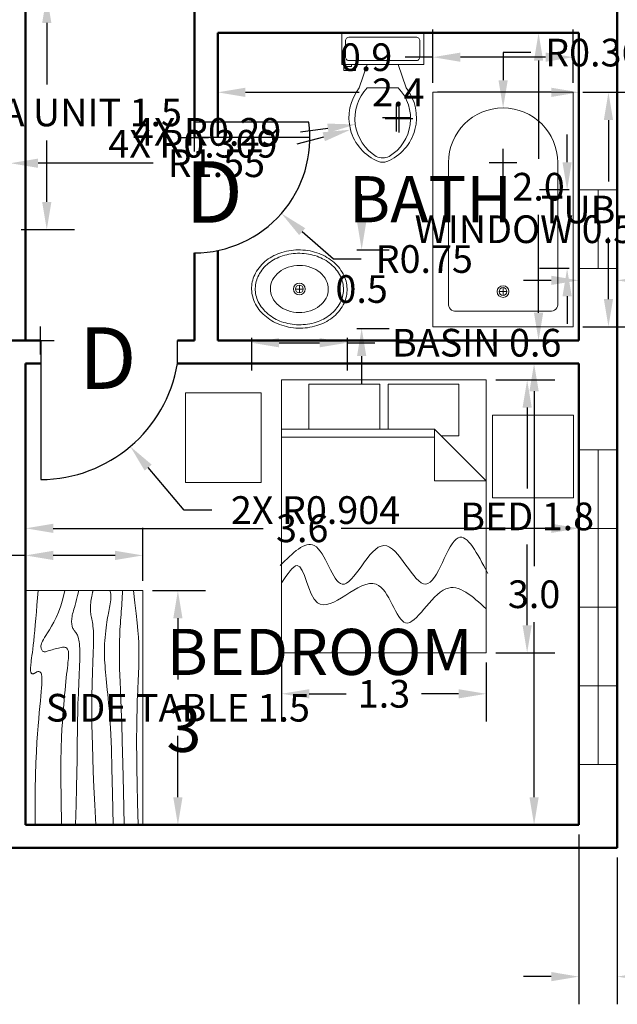
# Model space of a CAD drawing. Units: metres. Extents: x 3.9 to 21.3, y 24.8 to 56.5.
# Tile 2 of 6: x 11.9 to 15.8, y 24.8 to 31.2. Entities that reach past the tile are written whole.
import ezdxf

# ---------------------------------------------------------------- set-up
doc = ezdxf.new("R2010")
doc.units = ezdxf.units.M
doc.header["$MEASUREMENT"] = 0
for name, color, linetype, lineweight in [('A-AREA-IDEN', 3, 'Continuous', 25), ('A-FLOR-FIXT', 9, 'Continuous', 18), ('DIMENSIONS', 2, 'Continuous', 18), ('DOOR', 5, 'Continuous', 25), ('FURNITURE', 6, 'Continuous', 18), ('TEXT', 3, 'Continuous', 18), ('WALL', 1, 'Continuous', 50), ('WINDOW', 4, 'Continuous', 18)]:
    doc.layers.add(name, color=color, linetype=linetype, lineweight=lineweight)
doc.styles.get("Standard").update_dxf_attribs({"font": 'arial.ttf'})
doc.dimstyles.get("Standard").update_dxf_attribs({"dimtxt": 0.18, "dimasz": 0.18, "dimexe": 0.18, "dimexo": 0.0625, "dimgap": 0.09, "dimtad": 0, "dimtih": 1, "dimtoh": 1, "dimdec": 1, "dimzin": 0, "dimdsep": 46, "dimtxsty": 'Standard', "dimcen": 0.09, "dimadec": 0, "dimazin": 0, "dimtfac": 1, "dimtdec": 1, "dimtofl": 0, "dimtmove": 0, "dimatfit": 3, "dimfxl": 1, "dimtolj": 1, "dimtzin": 0, "dimarcsym": 0})

# ---------------------------------------------------------------- blocks, each defined once
blk = doc.blocks.new('Toilet - top')
for p, q in [((9.5, -6), (9.5, -2)), ((-10, -8.5), (-8, -8.5)), ((-10, -9.5), (-10, -8.5)), ((-7, -9.5), (-10, -9.5)), ((-8, -8.5), (-8, -8)), ((-7, -8), (-7, -9.5)), ((-4, -8), (-6, -14)), ((4, -8), (6, -14)), ((4, -14), (-4, -14))]:
    blk.add_line(p, q)
blk.add_lwpolyline([(10.5, -8), (10.5, 0), (-10.5, 0), (-10.5, -8)], close=True)
for points in [[(-9.5, -2), (-9.5, -6)], [(8.5, -1), (-8.5, -1)], [(-8.5, -7), (8.5, -7)]]:
    blk.add_lwpolyline(points)
for centre, radius, start, end in [((-8.62, -1.88), 0.884, 81.8699, 188.1301), ((8.62, -1.88), 0.884, 351.8699, 98.1301), ((-8.62, -6.12), 0.884, 171.8699, 278.1301), ((8.62, -6.12), 0.884, 261.8699, 8.1301), ((3.52, -21.58), 12.17, 141.4691, 247.9714), ((4.2, -21.82), 11.33, 136.3677, 238.9468), ((-3.52, -21.58), 12.17, 292.0284, 38.5307), ((-4.2, -21.82), 11.33, 301.053, 43.6321), ((0, -27.88), 4, 245.7318, 294.2682), ((0, -29), 4, 254.8605, 285.1395)]:
    blk.add_arc(centre, radius, start, end)
blk = doc.blocks.new('Bath Tub - 26 x 60 in.')
for p, q in [((9, -17), (9, -19)), ((8, -18), (10, -18))]:
    blk.add_line(p, q)
blk.add_lwpolyline([(0, -36), (0, 0), (60, 0), (60, -36)], close=True)
for points in [[(6, -4), (42, -4)], [(4, -30), (4, -6)], [(42, -32), (6, -32)]]:
    blk.add_lwpolyline(points)
for radius in [1.5, 1]:
    blk.add_circle((9, -18), radius)
for centre, radius, start, end in [((5.75, -5.75), 1.77, 81.8699, 188.1301), ((42, -18), 14, 270, 90), ((5.75, -30.25), 1.77, 171.8699, 278.1301)]:
    blk.add_arc(centre, radius, start, end)
blk = doc.blocks.new('Sink - Oval top')
for p, q in [((-1, 0), (1, 0)), ((0, 1), (0, -1))]:
    blk.add_line(p, q)
for points in [[(-12.23, 0.39, 0.117634), (-11.46, -3.36, 0.104469), (-8.88, -6.8, 0.090016), (-5.08, -9.07, 0.08192), (-0.32, -10.02, 0.08192), (4.49, -9.38, 0.090016), (8.42, -7.36, 0.104469), (11.22, -4.09, 0.117634), (12.23, -0.39, 0.117634), (11.46, 3.36, 0.104469), (8.88, 6.8, 0.090016), (5.08, 9.07, 0.08192), (0.32, 10.02, 0.08192), (-4.49, 9.38, 0.090016), (-8.42, 7.36, 0.104469), (-11.22, 4.09, 0.117634)], [(-11.29, 0.16, 0.118622), (-10.52, -3.25, 0.104678), (-8.07, -6.36, 0.089562), (-4.54, -8.37, 0.081185), (-0.13, -9.15, 0.081185), (4.3, -8.49, 0.089562), (7.89, -6.58, 0.104678), (10.42, -3.55, 0.118622), (11.29, -0.16, 0.118622), (10.52, 3.25, 0.104678), (8.07, 6.36, 0.089562), (4.54, 8.37, 0.081185), (0.13, 9.15, 0.081185), (-4.3, 8.49, 0.089562), (-7.89, 6.58, 0.104678), (-10.42, 3.55, 0.118622)], [(-7.42, 0.08, 0.118283), (-6.91, -2.17, 0.104607), (-5.29, -4.21, 0.089718), (-2.97, -5.53, 0.081436), (-0.07, -6.04, 0.081436), (2.84, -5.59, 0.089718), (5.2, -4.33, 0.104607), (6.86, -2.32, 0.118283), (7.42, -0.08, 0.118283), (6.91, 2.17, 0.104607), (5.29, 4.21, 0.089718), (2.97, 5.53, 0.081436), (0.07, 6.04, 0.081436), (-2.84, 5.59, 0.089718), (-5.2, 4.33, 0.104607), (-6.86, 2.32, 0.118283)]]:
    blk.add_lwpolyline(points, format="xyb", close=True)
for radius in [1.5, 1]:
    blk.add_circle((0, 0), radius)
blk = doc.blocks.new('Bed - Queen')
for p, q in [((0, -80.00003), (0, 0)), ((0, 0), (59.99999, 0)), ((59.99999, 0), (59.99999, -80.00003)), ((7.99999, -1.2), (28.79998, -1.2)), ((7.99999, -14.4), (7.99999, -1.2)), ((28.79998, -1.2), (28.79998, -14.4)), ((31.19999, -1.2), (51.99999, -1.2)), ((31.19999, -14.4), (31.19999, -1.2)), ((51.99999, -1.2), (51.99999, -16.4)), ((0, -14.4), (44.8, -14.4)), ((59.99999, -29.6), (44.8, -14.4)), ((44.8, -14.4), (44.8, -29.6)), ((44.8, -16.8), (0, -16.8)), ((51.99999, -16.4), (46.79936, -16.4)), ((44.8, -29.6), (59.99999, -29.6)), ((59.99999, -80.00003), (0, -80.00003))]:
    blk.add_line(p, q)
blk = doc.blocks.new('Table - Rectangular Woodgrain 60 x 30 in.')
for p, q in [((0, 0), (0, -30)), ((60, 0), (0, 0)), ((60, -30), (60, 0)), ((0, -30), (60, -30))]:
    blk.add_line(p, q)
for points in [[(0, -2.4), (4.8155, -2.418), (9.0302, -2.4688), (12.709, -2.5477), (15.9167, -2.65), (18.7181, -2.7711), (21.1781, -2.9063), (23.3616, -3.0508), (25.3333, -3.2), (27.1477, -3.3495), (28.8172, -3.4958), (30.3437, -3.636), (31.7291, -3.7667), (32.9756, -3.8849), (34.0849, -3.9875), (35.059, -4.0714), (35.9, -4.1334), (36.6114, -4.1711), (37.2041, -4.1854), (37.6906, -4.1779), (38.0833, -4.15), (38.3948, -4.1034), (38.6375, -4.0396), (38.8239, -3.9602), (38.9666, -3.8667), (39.0764, -3.7608), (39.1573, -3.6448), (39.2116, -3.521), (39.2416, -3.3917), (39.2498, -3.2593), (39.2385, -3.1261), (39.21, -2.9944), (39.1666, -2.8667), (39.111, -2.7447), (39.0468, -2.6281), (38.978, -2.5163), (38.9083, -2.4083), (38.8418, -2.3035), (38.7823, -2.201), (38.7337, -2.1001), (38.7, -2), (38.6844, -1.9003), (38.6875, -1.8021), (38.7094, -1.707), (38.75, -1.6167), (38.8094, -1.5326), (38.8875, -1.4563), (38.9844, -1.3893), (39.1, -1.3333), (39.2351, -1.2896), (39.3937, -1.2583), (39.5804, -1.2396), (39.8, -1.2333), (40.057, -1.2396), (40.3562, -1.2583), (40.7023, -1.2896), (41.1, -1.3333), (41.5547, -1.3895), (42.0755, -1.4573), (42.6721, -1.5361), (43.3542, -1.625), (44.1316, -1.7233), (45.014, -1.8302), (46.0114, -1.9449), (47.1333, -2.0667), (48.3862, -2.1947), (49.7625, -2.3281), (51.2513, -2.4663), (52.8416, -2.6083), (54.5226, -2.7535), (56.2833, -2.9011), (58.1127, -3.0501), (60, -3.2)], [(0, -9.2), (6.5759, -9.0858), (11.9385, -9.0365), (16.2527, -9.0418), (19.6833, -9.0917), (22.3952, -9.1759), (24.5531, -9.2844), (26.322, -9.4069), (27.8666, -9.5333), (29.3241, -9.6553), (30.7203, -9.7719), (32.0532, -9.8837), (33.3208, -9.9917), (34.5213, -10.0965), (35.6526, -10.199), (36.7128, -10.2999), (37.7, -10.4), (38.6129, -10.4996), (39.4531, -10.5969), (40.223, -10.6895), (40.925, -10.775), (41.5613, -10.8512), (42.1344, -10.9156), (42.6465, -10.966), (43.1, -11), (43.4976, -11.0158), (43.8437, -11.0136), (44.143, -10.9942), (44.4, -10.9583), (44.6195, -10.9069), (44.8062, -10.8406), (44.9648, -10.7603), (45.1, -10.6667), (45.2155, -10.5598), (45.3114, -10.4365), (45.3871, -10.2929), (45.4416, -10.125), (45.4743, -9.929), (45.4844, -9.7011), (45.4709, -9.4371), (45.4333, -9.1333), (45.3716, -8.7883), (45.2896, -8.4104), (45.1919, -8.0107), (45.0833, -7.6), (44.9685, -7.1893), (44.8521, -6.7896), (44.7388, -6.4117), (44.6333, -6.0667), (44.54, -5.7628), (44.4614, -5.4979), (44.4001, -5.2675), (44.3583, -5.0667), (44.3384, -4.8909), (44.3427, -4.7354), (44.3736, -4.5956), (44.4333, -4.4667), (44.5236, -4.3453), (44.6427, -4.2333), (44.7884, -4.1339), (44.9583, -4.05), (45.1501, -3.9849), (45.3614, -3.9417), (45.59, -3.9234), (45.8333, -3.9333), (46.0915, -3.9749), (46.3734, -4.0531), (46.6906, -4.1736), (47.0542, -4.3417), (47.4756, -4.5629), (47.9661, -4.8427), (48.5372, -5.1866), (49.2, -5.6), (49.9676, -6.0844), (50.8594, -6.625), (51.8965, -7.2031), (53.1, -7.8), (54.491, -8.3969), (56.0906, -8.975), (57.9199, -9.5156), (60, -10)], [(0, -12.8), (5.1847, -12.9322), (9.6213, -13.0323), (13.3963, -13.1059), (16.5958, -13.1583), (19.3063, -13.1952), (21.614, -13.2219), (23.6054, -13.2439), (25.3666, -13.2667), (26.9728, -13.2947), (28.4531, -13.3281), (29.8256, -13.3663), (31.1083, -13.4083), (32.3191, -13.4535), (33.476, -13.501), (34.597, -13.5501), (35.7, -13.6), (36.7984, -13.6497), (37.8875, -13.6979), (38.9578, -13.743), (40, -13.7833), (41.0047, -13.8174), (41.9625, -13.8438), (42.864, -13.8607), (43.7, -13.8667), (44.4631, -13.8604), (45.1552, -13.8417), (45.7801, -13.8104), (46.3416, -13.7667), (46.8439, -13.7104), (47.2906, -13.6417), (47.6858, -13.5604), (48.0333, -13.4667), (48.3375, -13.3608), (48.6042, -13.2448), (48.8396, -13.121), (49.05, -12.9917), (49.2417, -12.8593), (49.4208, -12.7261), (49.5937, -12.5944), (49.7667, -12.4667), (49.9452, -12.3451), (50.1323, -12.2313), (50.3303, -12.1268), (50.5416, -12.0333), (50.7686, -11.9524), (51.0135, -11.8854), (51.2788, -11.8341), (51.5666, -11.8), (51.8785, -11.7843), (52.2116, -11.7865), (52.562, -11.8059), (52.926, -11.8417), (53.2998, -11.8931), (53.6795, -11.9594), (54.0614, -12.0397), (54.4416, -12.1333), (54.8223, -12.2401), (55.2293, -12.3625), (55.6942, -12.5037), (56.2489, -12.6667), (56.9251, -12.8547), (57.7545, -13.0708), (58.7689, -13.3182), (60, -13.6)], [(0, -18), (5.124, -17.7273), (9.6609, -17.5057), (13.6705, -17.3303), (17.2125, -17.1958), (20.3467, -17.0973), (23.1328, -17.0297), (25.6307, -16.9878), (27.9, -16.9667), (29.9928, -16.9617), (31.9302, -16.9703), (33.7254, -16.9907), (35.3917, -17.0208), (36.9423, -17.0588), (38.3906, -17.1026), (39.7499, -17.1503), (41.0333, -17.2), (42.2519, -17.2496), (43.4073, -17.2969), (44.4986, -17.3395), (45.525, -17.375), (46.4858, -17.4012), (47.3802, -17.4156), (48.2074, -17.416), (48.9667, -17.4), (49.6583, -17.3662), (50.2872, -17.3167), (50.8595, -17.2547), (51.3812, -17.1833), (51.8584, -17.1057), (52.2971, -17.025), (52.7034, -16.9443), (53.0833, -16.8667), (53.443, -16.7951), (53.789, -16.7313), (54.128, -16.6768), (54.4666, -16.6334), (54.8115, -16.6024), (55.1693, -16.5854), (55.5465, -16.5841), (55.95, -16.6), (56.3828, -16.6337), (56.8346, -16.6823), (57.2915, -16.7418), (57.7396, -16.8084), (58.165, -16.878), (58.5539, -16.9469), (58.8924, -17.0111), (59.1666, -17.0667), (59.3679, -17.1107), (59.5078, -17.1438), (59.6032, -17.1675), (59.6708, -17.1833), (59.7275, -17.193), (59.7901, -17.1979), (59.8753, -17.1998), (60, -17.2)], [(0, -22.4), (8.0098, -22.2501), (14.4094, -22.1011), (19.4168, -21.9535), (23.25, -21.8083), (26.1269, -21.6663), (28.2656, -21.5281), (29.884, -21.3947), (31.2, -21.2667), (32.3967, -21.1448), (33.5172, -21.0292), (34.5697, -20.9198), (35.5625, -20.8167), (36.5037, -20.7198), (37.4015, -20.6292), (38.2642, -20.5448), (39.1, -20.4667), (39.9164, -20.3951), (40.7187, -20.3313), (41.5117, -20.2768), (42.3, -20.2333), (43.0883, -20.2024), (43.8812, -20.1854), (44.6836, -20.1841), (45.5, -20.2), (46.3328, -20.234), (47.1747, -20.2844), (48.0163, -20.3488), (48.8479, -20.425), (49.66, -20.5106), (50.4429, -20.6031), (51.1872, -20.7004), (51.8833, -20.8), (52.5246, -20.8999), (53.1166, -20.9995), (53.6681, -21.0983), (54.1875, -21.1958), (54.6834, -21.2919), (55.1646, -21.3859), (55.6394, -21.4777), (56.1167, -21.5667), (56.6028, -21.6515), (57.0961, -21.7266), (57.5929, -21.7852), (58.0896, -21.8208), (58.5823, -21.8268), (59.0674, -21.7964), (59.5412, -21.723), (60, -21.6)], [(0, -25.2), (8.6355, -25.0504), (15.7026, -24.9031), (21.4049, -24.7606), (25.9458, -24.625), (29.529, -24.4988), (32.3578, -24.3844), (34.6359, -24.284), (36.5667, -24.2), (38.3213, -24.1341), (39.9417, -24.0854), (41.437, -24.0523), (42.8167, -24.0333), (44.0901, -24.0268), (45.2667, -24.0313), (46.3557, -24.0451), (47.3667, -24.0667), (48.309, -24.0947), (49.1928, -24.1287), (50.0284, -24.168), (50.826, -24.2125), (51.5959, -24.2617), (52.3483, -24.3151), (53.0935, -24.3725), (53.8417, -24.4334), (54.6009, -24.497), (55.3699, -24.561), (56.1454, -24.6226), (56.9239, -24.6792), (57.7021, -24.7279), (58.4764, -24.7662), (59.2435, -24.7911), (60, -24.8)], [(0, -28.8), (5.6867, -28.6681), (10.45, -28.5698), (14.407, -28.5012), (17.675, -28.4584), (20.3711, -28.4374), (22.6125, -28.4344), (24.5164, -28.4455), (26.2, -28.4667), (27.762, -28.4947), (29.2276, -28.5281), (30.6033, -28.5663), (31.8958, -28.6084), (33.1118, -28.6535), (34.2578, -28.7011), (35.3405, -28.7501), (36.3666, -28.8), (37.3443, -28.8497), (38.288, -28.8974), (39.2137, -28.9412), (40.1375, -28.9792), (41.0753, -29.0093), (42.0432, -29.0297), (43.0572, -29.0384), (44.1333, -29.0333), (45.2936, -29.0114), (46.5843, -28.9641), (48.0579, -28.8816), (49.7666, -28.7542), (51.7629, -28.5721), (54.0989, -28.3255), (56.8272, -28.0048), (60, -27.6)]]:
    blk.add_lwpolyline(points)
blk = doc.blocks.new('*D21')
at = {"layer": 'Defpoints', "color": 0, "transparency": 16777216}
for p in [(15.7571, 38.8951), (15.7571, 25.8451), (17.2883, 25.8451)]:
    blk.add_point(p, dxfattribs=at)
at = {"layer": 'DIMENSIONS', "color": 0, "lineweight": -2, "transparency": 16777216}
for p, q in [((15.8196, 38.8951), (17.4683, 38.8951)), ((17.2883, 38.7151), (17.2883, 32.8688)), ((17.2883, 26.0251), (17.2883, 31.8713)), ((15.8196, 25.8451), (17.4683, 25.8451))]:
    blk.add_line(p, q, dxfattribs=at)
at = {"layer": 'DIMENSIONS', "color": 0, "transparency": 16777216}
for points in [[(17.2583, 38.7151), (17.3183, 38.7151), (17.2883, 38.8951)], [(17.2583, 26.0251), (17.3183, 26.0251), (17.2883, 25.8451)]]:
    blk.add_solid(points, dxfattribs=at)
at = {"layer": 'DIMENSIONS', "color": 0, "transparency": 16777216, "insert": (17.2883, 32.3701), "char_height": 0.18, "attachment_point": 5}
blk.add_mtext('\\A1;{\\H4.44444x;13.1}', dxfattribs=at)
blk = doc.blocks.new('*D30')
at = {"layer": 'Defpoints', "color": 0, "transparency": 16777216}
for p in [(13.8962, 31.1451), (13.9549, 29.1451), (15.2447, 29.1451)]:
    blk.add_point(p, dxfattribs=at)
at = {"layer": 'DIMENSIONS', "color": 0, "lineweight": -2, "transparency": 16777216}
for p, q in [((13.9587, 31.1451), (15.4247, 31.1451)), ((15.2447, 30.9651), (15.2447, 30.327)), ((15.2447, 29.3251), (15.2447, 29.9632)), ((14.0174, 29.1451), (15.4247, 29.1451))]:
    blk.add_line(p, q, dxfattribs=at)
at = {"layer": 'DIMENSIONS', "color": 0, "transparency": 16777216}
for points in [[(15.2147, 30.9651), (15.2747, 30.9651), (15.2447, 31.1451)], [(15.2147, 29.3251), (15.2747, 29.3251), (15.2447, 29.1451)]]:
    blk.add_solid(points, dxfattribs=at)
at = {"layer": 'DIMENSIONS', "color": 0, "transparency": 16777216, "insert": (15.2447, 30.1451), "char_height": 0.18, "attachment_point": 5}
blk.add_mtext('\\A1;2.0', dxfattribs=at)
blk = doc.blocks.new('*D31')
at = {"layer": 'Defpoints', "color": 0, "transparency": 16777216}
for p in [(13.1571, 31.1451), (15.5071, 31.1451), (15.5071, 30.7589)]:
    blk.add_point(p, dxfattribs=at)
at = {"layer": 'DIMENSIONS', "color": 0, "lineweight": -2, "transparency": 16777216}
for p, q in [((13.1571, 31.0826), (13.1571, 30.5789)), ((15.5071, 31.0826), (15.5071, 30.5789)), ((13.3371, 30.7589), (14.0771, 30.7589)), ((15.3271, 30.7589), (14.5871, 30.7589))]:
    blk.add_line(p, q, dxfattribs=at)
at = {"layer": 'DIMENSIONS', "color": 0, "transparency": 16777216}
for points in [[(13.3371, 30.7889), (13.3371, 30.7289), (13.1571, 30.7589)], [(15.3271, 30.7889), (15.3271, 30.7289), (15.5071, 30.7589)]]:
    blk.add_solid(points, dxfattribs=at)
at = {"layer": 'DIMENSIONS', "color": 0, "transparency": 16777216, "insert": (14.3321, 30.7589), "char_height": 0.18, "attachment_point": 5}
blk.add_mtext('\\A1;2.4', dxfattribs=at)
blk = doc.blocks.new('*D32')
at = {"layer": 'Defpoints', "color": 0, "transparency": 16777216}
for p in [(15.5071, 28.9951), (15.2156, 25.9951), (15.5071, 25.9951)]:
    blk.add_point(p, dxfattribs=at)
at = {"layer": 'DIMENSIONS', "color": 0, "lineweight": -2, "transparency": 16777216}
for p, q in [((15.4446, 28.9951), (15.0356, 28.9951)), ((15.2156, 28.8151), (15.2156, 27.677)), ((15.2156, 26.1751), (15.2156, 27.3131)), ((15.4446, 25.9951), (15.0356, 25.9951))]:
    blk.add_line(p, q, dxfattribs=at)
at = {"layer": 'DIMENSIONS', "color": 0, "transparency": 16777216}
for points in [[(15.1856, 28.8151), (15.2456, 28.8151), (15.2156, 28.9951)], [(15.1856, 26.1751), (15.2456, 26.1751), (15.2156, 25.9951)]]:
    blk.add_solid(points, dxfattribs=at)
at = {"layer": 'DIMENSIONS', "color": 0, "transparency": 16777216, "insert": (15.2156, 27.4951), "char_height": 0.18, "attachment_point": 5}
blk.add_mtext('\\A1;3.0', dxfattribs=at)
blk = doc.blocks.new('*D33')
at = {"layer": 'Defpoints', "color": 0, "transparency": 16777216}
for p in [(11.9071, 27.9939), (15.5071, 27.9237), (15.5071, 27.9237)]:
    blk.add_point(p, dxfattribs=at)
at = {"layer": 'DIMENSIONS', "color": 0, "lineweight": -2, "transparency": 16777216}
for p, q in [((15.5071, 27.9862), (15.5071, 28.1037)), ((11.9071, 27.9314), (11.9071, 27.7437)), ((12.0871, 27.9237), (13.4534, 27.9237)), ((15.3271, 27.9237), (13.9609, 27.9237))]:
    blk.add_line(p, q, dxfattribs=at)
at = {"layer": 'DIMENSIONS', "color": 0, "transparency": 16777216}
for points in [[(12.0871, 27.9537), (12.0871, 27.8937), (11.9071, 27.9237)], [(15.3271, 27.9537), (15.3271, 27.8937), (15.5071, 27.9237)]]:
    blk.add_solid(points, dxfattribs=at)
at = {"layer": 'DIMENSIONS', "color": 0, "transparency": 16777216, "insert": (13.7071, 27.9237), "char_height": 0.18, "attachment_point": 5}
blk.add_mtext('\\A1;3.6', dxfattribs=at)
blk = doc.blocks.new('WIN-4-LIGHT-2046')
for p, q in [((0.5115, -0.125), (0, -0.125)), ((0.5115, -0.125), (1.0231, -0.125)), ((1.5346, -0.125), (1.0231, -0.125)), ((1.5346, -0.125), (2.0462, -0.125))]:
    blk.add_line(p, q)
for points in [[(0.5115, 0), (0, 0), (0, -0.25), (0.5115, -0.25)], [(0.5115, 0), (1.0231, 0), (1.0231, -0.25), (0.5115, -0.25)], [(1.5346, 0), (1.0231, 0), (1.0231, -0.25), (1.5346, -0.25)], [(1.5346, 0), (2.0462, 0), (2.0462, -0.25), (1.5346, -0.25)]]:
    blk.add_lwpolyline(points, close=True)
blk = doc.blocks.new('WIN-1-LIGHT-512')
blk.add_line((0, -0.125), (0.5115, -0.125))
blk.add_lwpolyline([(0, 0), (0.5115, 0), (0.5115, -0.25), (0, -0.25)], close=True)
blk = doc.blocks.new('*D43')
at = {"layer": 'Defpoints', "color": 0, "transparency": 16777216}
for p in [(14.9043, 28.8887), (15.1705, 28.8887), (14.9043, 27.1139)]:
    blk.add_point(p, dxfattribs=at)
at = {"layer": 'DIMENSIONS', "color": 0, "lineweight": -2, "transparency": 16777216}
for p, q in [((14.9668, 28.8887), (15.3505, 28.8887)), ((15.1705, 28.7087), (15.1705, 28.1832)), ((15.1705, 27.2939), (15.1705, 27.8194)), ((14.9668, 27.1139), (15.3505, 27.1139))]:
    blk.add_line(p, q, dxfattribs=at)
at = {"layer": 'DIMENSIONS', "color": 0, "transparency": 16777216}
for points in [[(15.1405, 28.7087), (15.2005, 28.7087), (15.1705, 28.8887)], [(15.1405, 27.2939), (15.2005, 27.2939), (15.1705, 27.1139)]]:
    blk.add_solid(points, dxfattribs=at)
at = {"layer": 'DIMENSIONS', "color": 0, "transparency": 16777216, "insert": (15.1705, 28.0013), "char_height": 0.18, "attachment_point": 5}
blk.add_mtext('\\A1;BED 1.8', dxfattribs=at)
blk = doc.blocks.new('*D44')
at = {"layer": 'Defpoints', "color": 0, "transparency": 16777216}
for p in [(13.5732, 27.1139), (14.9043, 27.1139), (14.9043, 26.8477)]:
    blk.add_point(p, dxfattribs=at)
at = {"layer": 'DIMENSIONS', "color": 0, "lineweight": -2, "transparency": 16777216}
for p, q in [((13.5732, 27.0514), (13.5732, 26.6677)), ((14.9043, 27.0514), (14.9043, 26.6677)), ((13.7532, 26.8477), (13.9934, 26.8477)), ((14.7243, 26.8477), (14.4841, 26.8477))]:
    blk.add_line(p, q, dxfattribs=at)
at = {"layer": 'DIMENSIONS', "color": 0, "transparency": 16777216}
for points in [[(13.7532, 26.8777), (13.7532, 26.8177), (13.5732, 26.8477)], [(14.7243, 26.8777), (14.7243, 26.8177), (14.9043, 26.8477)]]:
    blk.add_solid(points, dxfattribs=at)
at = {"layer": 'DIMENSIONS', "color": 0, "transparency": 16777216, "insert": (14.2388, 26.8477), "char_height": 0.18, "attachment_point": 5}
blk.add_mtext('\\A1;1.3', dxfattribs=at)
blk = doc.blocks.new('*D47')
at = {"layer": 'Defpoints', "color": 0, "transparency": 16777216}
for p in [(15.5071, 30.1245), (15.4304, 29.6129), (15.5071, 29.6129)]:
    blk.add_point(p, dxfattribs=at)
at = {"layer": 'DIMENSIONS', "color": 0, "lineweight": -2, "transparency": 16777216}
for p, q in [((15.4304, 30.3045), (15.4304, 30.4845)), ((15.4446, 30.1245), (15.2504, 30.1245)), ((15.4446, 29.6129), (15.2504, 29.6129)), ((15.4304, 29.4329), (15.4304, 29.2529))]:
    blk.add_line(p, q, dxfattribs=at)
at = {"layer": 'DIMENSIONS', "color": 0, "transparency": 16777216}
for points in [[(15.4004, 30.3045), (15.4604, 30.3045), (15.4304, 30.1245)], [(15.4004, 29.4329), (15.4604, 29.4329), (15.4304, 29.6129)]]:
    blk.add_solid(points, dxfattribs=at)
at = {"layer": 'DIMENSIONS', "color": 0, "transparency": 16777216, "insert": (15.4304, 29.8687), "char_height": 0.18, "attachment_point": 5}
blk.add_mtext('\\A1;WINDOW 0.5 TYP.', dxfattribs=at)
blk = doc.blocks.new('*D48')
at = {"layer": 'Defpoints', "color": 0, "transparency": 16777216}
for p in [(15.5071, 29.6129), (15.7571, 29.6129), (15.7571, 29.5362)]:
    blk.add_point(p, dxfattribs=at)
at = {"layer": 'DIMENSIONS', "color": 0, "lineweight": -2, "transparency": 16777216}
for p, q in [((15.3271, 29.5362), (15.1471, 29.5362)), ((15.5071, 29.5504), (15.5071, 29.3562)), ((15.7571, 29.5504), (15.7571, 29.3562)), ((15.9371, 29.5362), (16.1171, 29.5362))]:
    blk.add_line(p, q, dxfattribs=at)
at = {"layer": 'DIMENSIONS', "color": 0, "transparency": 16777216}
for points in [[(15.3271, 29.5662), (15.3271, 29.5062), (15.5071, 29.5362)], [(15.9371, 29.5662), (15.9371, 29.5062), (15.7571, 29.5362)]]:
    blk.add_solid(points, dxfattribs=at)
at = {"layer": 'DIMENSIONS', "color": 0, "transparency": 16777216, "insert": (16.6801, 29.5362), "char_height": 0.18, "attachment_point": 5}
blk.add_mtext('\\A1;0.3 TYP.', dxfattribs=at)
blk = doc.blocks.new('*D59')
at = {"layer": 'Defpoints', "color": 0, "transparency": 16777216}
for p in [(11.8164, 31.3903), (12.045, 31.3903), (11.8164, 29.8663)]:
    blk.add_point(p, dxfattribs=at)
at = {"layer": 'DIMENSIONS', "color": 0, "lineweight": -2, "transparency": 16777216}
for p, q in [((11.8789, 31.3903), (12.225, 31.3903)), ((12.045, 31.2103), (12.045, 30.8102)), ((12.045, 30.0463), (12.045, 30.4464)), ((11.8789, 29.8663), (12.225, 29.8663))]:
    blk.add_line(p, q, dxfattribs=at)
at = {"layer": 'DIMENSIONS', "color": 0, "transparency": 16777216}
for points in [[(12.015, 31.2103), (12.075, 31.2103), (12.045, 31.3903)], [(12.015, 30.0463), (12.075, 30.0463), (12.045, 29.8663)]]:
    blk.add_solid(points, dxfattribs=at)
at = {"layer": 'DIMENSIONS', "color": 0, "transparency": 16777216, "insert": (12.045, 30.6283), "char_height": 0.18, "attachment_point": 5}
blk.add_mtext('\\A1;MEDIA UNIT 1.5', dxfattribs=at)
blk = doc.blocks.new('*D67')
at = {"layer": 'Defpoints', "color": 0, "transparency": 16777216}
for p in [(15.4709, 30.7589), (15.6995, 30.7589), (15.4709, 29.2349)]:
    blk.add_point(p, dxfattribs=at)
at = {"layer": 'DIMENSIONS', "color": 0, "lineweight": -2, "transparency": 16777216}
for p, q in [((15.5334, 30.7589), (15.8795, 30.7589)), ((15.6995, 30.5789), (15.6995, 30.1788)), ((15.6995, 29.4149), (15.6995, 29.8149)), ((15.5334, 29.2349), (15.8795, 29.2349))]:
    blk.add_line(p, q, dxfattribs=at)
at = {"layer": 'DIMENSIONS', "color": 0, "transparency": 16777216}
for points in [[(15.6695, 30.5789), (15.7295, 30.5789), (15.6995, 30.7589)], [(15.6695, 29.4149), (15.7295, 29.4149), (15.6995, 29.2349)]]:
    blk.add_solid(points, dxfattribs=at)
at = {"layer": 'DIMENSIONS', "color": 0, "transparency": 16777216, "insert": (15.6995, 29.9969), "char_height": 0.18, "attachment_point": 5}
blk.add_mtext('\\A1;TUB 1.5', dxfattribs=at)
blk = doc.blocks.new('*D68')
at = {"layer": 'Defpoints', "color": 0, "transparency": 16777216}
for p in [(14.5565, 30.9875), (14.5565, 30.7589), (15.4709, 30.7589)]:
    blk.add_point(p, dxfattribs=at)
at = {"layer": 'DIMENSIONS', "color": 0, "lineweight": -2, "transparency": 16777216}
for p, q in [((14.5565, 30.8214), (14.5565, 31.1675)), ((15.4709, 30.8214), (15.4709, 31.1675)), ((14.5565, 30.9875), (14.3765, 30.9875)), ((15.2909, 30.9875), (14.7365, 30.9875))]:
    blk.add_line(p, q, dxfattribs=at)
at = {"layer": 'DIMENSIONS', "color": 0, "transparency": 16777216}
for points in [[(14.7365, 31.0175), (14.7365, 30.9575), (14.5565, 30.9875)], [(15.2909, 31.0175), (15.2909, 30.9575), (15.4709, 30.9875)]]:
    blk.add_solid(points, dxfattribs=at)
at = {"layer": 'DIMENSIONS', "color": 0, "transparency": 16777216, "insert": (14.1225, 30.9875), "char_height": 0.18, "attachment_point": 5}
blk.add_mtext('\\A1;0.9', dxfattribs=at)
blk = doc.blocks.new('*D69')
at = {"layer": 'Defpoints', "color": 0, "transparency": 16777216}
for p in [(13.3765, 29.2242), (14.0001, 29.2242), (14.0001, 29.1307)]:
    blk.add_point(p, dxfattribs=at)
at = {"layer": 'DIMENSIONS', "color": 0, "lineweight": -2, "transparency": 16777216}
for p, q in [((13.3765, 29.1617), (13.3765, 28.9507)), ((14.0001, 29.1617), (14.0001, 28.9507)), ((13.5565, 29.1307), (13.8201, 29.1307)), ((14.0001, 29.1307), (14.1801, 29.1307))]:
    blk.add_line(p, q, dxfattribs=at)
at = {"layer": 'DIMENSIONS', "color": 0, "transparency": 16777216}
for points in [[(13.5565, 29.1607), (13.5565, 29.1007), (13.3765, 29.1307)], [(13.8201, 29.1607), (13.8201, 29.1007), (14.0001, 29.1307)]]:
    blk.add_solid(points, dxfattribs=at)
at = {"layer": 'DIMENSIONS', "color": 0, "transparency": 16777216, "insert": (14.8421, 29.1307), "char_height": 0.18, "attachment_point": 5}
blk.add_mtext('\\A1;BASIN 0.6', dxfattribs=at)
blk = doc.blocks.new('*D70')
at = {"layer": 'Defpoints', "color": 0, "transparency": 16777216}
for p in [(14.0001, 29.7357), (14.0936, 29.7357), (14.0001, 29.2242)]:
    blk.add_point(p, dxfattribs=at)
at = {"layer": 'DIMENSIONS', "color": 0, "lineweight": -2, "transparency": 16777216}
for p, q in [((14.0936, 29.9157), (14.0936, 30.0957)), ((14.0626, 29.7357), (14.2736, 29.7357)), ((14.0626, 29.2242), (14.2736, 29.2242)), ((14.0936, 29.0442), (14.0936, 28.8642))]:
    blk.add_line(p, q, dxfattribs=at)
at = {"layer": 'DIMENSIONS', "color": 0, "transparency": 16777216}
for points in [[(14.0636, 29.9157), (14.1236, 29.9157), (14.0936, 29.7357)], [(14.0636, 29.0442), (14.1236, 29.0442), (14.0936, 29.2242)]]:
    blk.add_solid(points, dxfattribs=at)
at = {"layer": 'DIMENSIONS', "color": 0, "transparency": 16777216, "insert": (14.0936, 29.4799), "char_height": 0.18, "attachment_point": 5}
blk.add_mtext('\\A1;0.5', dxfattribs=at)
blk = doc.blocks.new('*D71')
at = {"layer": 'Defpoints', "color": 0, "transparency": 16777216}
for p in [(12.6694, 27.519), (12.898, 27.519), (12.6694, 25.995)]:
    blk.add_point(p, dxfattribs=at)
at = {"layer": 'DIMENSIONS', "color": 0, "lineweight": -2, "transparency": 16777216}
for p, q in [((12.7319, 27.519), (13.078, 27.519)), ((12.898, 27.339), (12.898, 26.9401)), ((12.898, 26.175), (12.898, 26.5739)), ((12.7319, 25.995), (13.078, 25.995))]:
    blk.add_line(p, q, dxfattribs=at)
at = {"layer": 'DIMENSIONS', "color": 0, "transparency": 16777216}
for points in [[(12.868, 27.339), (12.928, 27.339), (12.898, 27.519)], [(12.868, 26.175), (12.928, 26.175), (12.898, 25.995)]]:
    blk.add_solid(points, dxfattribs=at)
at = {"layer": 'DIMENSIONS', "color": 0, "transparency": 16777216, "insert": (12.898, 26.757), "char_height": 0.18, "attachment_point": 5}
blk.add_mtext('\\A1;SIDE TABLE 1.5', dxfattribs=at)
blk = doc.blocks.new('*D72')
at = {"layer": 'Defpoints', "color": 0, "transparency": 16777216}
for p in [(11.9074, 27.7476), (11.9074, 27.519), (12.6694, 27.519)]:
    blk.add_point(p, dxfattribs=at)
at = {"layer": 'DIMENSIONS', "color": 0, "lineweight": -2, "transparency": 16777216}
for p, q in [((11.9074, 27.5815), (11.9074, 27.9276)), ((12.6694, 27.5815), (12.6694, 27.9276)), ((11.9074, 27.7476), (11.7274, 27.7476)), ((12.4894, 27.7476), (12.0874, 27.7476))]:
    blk.add_line(p, q, dxfattribs=at)
at = {"layer": 'DIMENSIONS', "color": 0, "transparency": 16777216}
for points in [[(12.0874, 27.7776), (12.0874, 27.7176), (11.9074, 27.7476)], [(12.4894, 27.7776), (12.4894, 27.7176), (12.6694, 27.7476)]]:
    blk.add_solid(points, dxfattribs=at)
at = {"layer": 'DIMENSIONS', "color": 0, "transparency": 16777216, "insert": (11.4733, 27.7476), "char_height": 0.18, "attachment_point": 5}
blk.add_mtext('\\A1;0.8', dxfattribs=at)
blk = doc.blocks.new('*D94')
at = {"layer": 'Defpoints', "color": 0, "transparency": 16777216}
for p in [(15.5071, 25.9951), (15.7571, 25.8451), (15.7571, 25.0086)]:
    blk.add_point(p, dxfattribs=at)
at = {"layer": 'DIMENSIONS', "color": 0, "lineweight": -2, "transparency": 16777216}
for p, q in [((15.5071, 25.9326), (15.5071, 24.8286)), ((15.7571, 25.7826), (15.7571, 24.8286)), ((15.3271, 25.0086), (15.1471, 25.0086)), ((15.9371, 25.0086), (16.1171, 25.0086))]:
    blk.add_line(p, q, dxfattribs=at)
at = {"layer": 'DIMENSIONS', "color": 0, "transparency": 16777216}
for points in [[(15.3271, 25.0386), (15.3271, 24.9786), (15.5071, 25.0086)], [(15.9371, 25.0386), (15.9371, 24.9786), (15.7571, 25.0086)]]:
    blk.add_solid(points, dxfattribs=at)
at = {"layer": 'DIMENSIONS', "color": 0, "transparency": 16777216, "insert": (16.4416, 25.0086), "char_height": 0.18, "attachment_point": 5}
blk.add_mtext('\\A1;0.25', dxfattribs=at)
blk = doc.blocks.new('*D104')
at = {"layer": 'Defpoints', "color": 0, "transparency": 16777216}
for p in [(12.0032, 29.1451), (12.5881, 28.4559)]:
    blk.add_point(p, dxfattribs=at)
at = {"layer": 'DIMENSIONS', "color": 0, "lineweight": -2, "transparency": 16777216}
for p, q in [((12.0032, 29.0551), (12.0032, 29.2351)), ((11.9132, 29.1451), (12.0932, 29.1451)), ((12.9391, 28.0424), (12.7046, 28.3186)), ((13.1191, 28.0424), (12.9391, 28.0424))]:
    blk.add_line(p, q, dxfattribs=at)
at = {"layer": 'DIMENSIONS', "color": 0, "transparency": 16777216}
blk.add_solid([(12.7275, 28.3381), (12.6817, 28.2992), (12.5881, 28.4559)], dxfattribs=at)
at = {"layer": 'DIMENSIONS', "color": 0, "transparency": 16777216, "insert": (13.7935, 28.0424), "char_height": 0.18, "attachment_point": 5}
blk.add_mtext('\\A1;2X R0.904', dxfattribs=at)
blk = doc.blocks.new('*D105')
at = {"layer": 'Defpoints', "color": 0, "transparency": 16777216}
for p in [(13.0071, 30.4651), (13.5717, 29.9713)]:
    blk.add_point(p, dxfattribs=at)
at = {"layer": 'DIMENSIONS', "color": 0, "lineweight": -2, "transparency": 16777216}
for p, q in [((13.0071, 30.3751), (13.0071, 30.5551)), ((12.9171, 30.4651), (13.0971, 30.4651)), ((13.9104, 29.675), (13.7071, 29.8528)), ((14.0904, 29.675), (13.9104, 29.675))]:
    blk.add_line(p, q, dxfattribs=at)
at = {"layer": 'DIMENSIONS', "color": 0, "transparency": 16777216}
blk.add_solid([(13.7269, 29.8754), (13.6874, 29.8302), (13.5717, 29.9713)], dxfattribs=at)
at = {"layer": 'DIMENSIONS', "color": 0, "transparency": 16777216, "insert": (14.501, 29.675), "char_height": 0.18, "attachment_point": 5}
blk.add_mtext('\\A1;R0.75', dxfattribs=at)
blk = doc.blocks.new('*D111')
at = {"layer": 'Defpoints', "color": 0, "transparency": 16777216}
for p in [(10.2586, 30.2981), (11.808, 30.298)]:
    blk.add_point(p, dxfattribs=at)
at = {"layer": 'DIMENSIONS', "color": 0, "lineweight": -2, "transparency": 16777216}
for p, q in [((10.2586, 30.2081), (10.2586, 30.3881)), ((10.1686, 30.2981), (10.3486, 30.2981)), ((12.7376, 30.2979), (11.988, 30.298))]:
    blk.add_line(p, q, dxfattribs=at)
at = {"layer": 'DIMENSIONS', "color": 0, "transparency": 16777216}
blk.add_solid([(11.988, 30.328), (11.988, 30.268), (11.808, 30.298)], dxfattribs=at)
at = {"layer": 'DIMENSIONS', "color": 0, "transparency": 16777216, "insert": (13.1482, 30.2979), "char_height": 0.18, "attachment_point": 5}
blk.add_mtext('\\A1;R1.55', dxfattribs=at)
blk = doc.blocks.new('*D112')
at = {"layer": 'Defpoints', "color": 0, "transparency": 16777216}
for p in [(15.014, 30.6573), (15.0137, 30.3017)]:
    blk.add_point(p, dxfattribs=at)
at = {"layer": 'DIMENSIONS', "color": 0, "lineweight": -2, "transparency": 16777216}
for p, q in [((15.0143, 31.0173), (15.0141, 30.8373)), ((15.1943, 31.0173), (15.0143, 31.0173)), ((15.0137, 30.2117), (15.0137, 30.3917)), ((14.9237, 30.3017), (15.1037, 30.3017))]:
    blk.add_line(p, q, dxfattribs=at)
at = {"layer": 'DIMENSIONS', "color": 0, "transparency": 16777216}
blk.add_solid([(14.9841, 30.8373), (15.0441, 30.8372), (15.014, 30.6573)], dxfattribs=at)
at = {"layer": 'DIMENSIONS', "color": 0, "transparency": 16777216, "insert": (15.6041, 31.0173), "char_height": 0.18, "attachment_point": 5}
blk.add_mtext('\\A1;R0.36', dxfattribs=at)
blk = doc.blocks.new('*D113')
at = {"layer": 'Defpoints', "color": 0, "transparency": 16777216}
for p in [(14.3201, 30.5948), (14.0212, 30.5161)]:
    blk.add_point(p, dxfattribs=at)
at = {"layer": 'DIMENSIONS', "color": 0, "lineweight": -2, "transparency": 16777216}
for p, q in [((14.3201, 30.5048), (14.3201, 30.6848)), ((14.2301, 30.5948), (14.4101, 30.5948)), ((13.6731, 30.4244), (13.8471, 30.4702))]:
    blk.add_line(p, q, dxfattribs=at)
at = {"layer": 'DIMENSIONS', "color": 0, "transparency": 16777216}
blk.add_solid([(13.8395, 30.4992), (13.8548, 30.4412), (14.0212, 30.5161)], dxfattribs=at)
at = {"layer": 'DIMENSIONS', "color": 0, "transparency": 16777216, "insert": (12.996, 30.4244), "char_height": 0.18, "attachment_point": 5}
blk.add_mtext('\\A1;4X R0.309', dxfattribs=at)
blk = doc.blocks.new('*D114')
at = {"layer": 'Defpoints', "color": 0, "transparency": 16777216}
for p in [(14.0523, 30.55), (14.3374, 30.5887)]:
    blk.add_point(p, dxfattribs=at)
at = {"layer": 'DIMENSIONS', "color": 0, "lineweight": -2, "transparency": 16777216}
for p, q in [((14.3374, 30.4987), (14.3374, 30.6787)), ((14.2474, 30.5887), (14.4274, 30.5887)), ((13.6955, 30.5016), (13.8739, 30.5258))]:
    blk.add_line(p, q, dxfattribs=at)
at = {"layer": 'DIMENSIONS', "color": 0, "transparency": 16777216}
blk.add_solid([(13.8699, 30.5556), (13.8779, 30.4961), (14.0523, 30.55)], dxfattribs=at)
at = {"layer": 'DIMENSIONS', "color": 0, "transparency": 16777216, "insert": (13.0884, 30.5016), "char_height": 0.18, "attachment_point": 5}
blk.add_mtext('\\A1;4X R0.29', dxfattribs=at)

msp = doc.modelspace()

# ---------------------------------------------------------------- linework, layer by layer
at = {"layer": 'DOOR'}
for p, q in [((13.7504, 30.5651), (13.0071, 30.5651)), ((13.7571, 30.4651), (13.0071, 30.4651)), ((12.0071, 29.1451), (12.0071, 28.2411)), ((12.8946, 28.9951), (12.8946, 29.1451))]:
    msp.add_line(p, q, dxfattribs=at)
for centre, radius, start, end in [((13.0071, 30.4651), 0.75, 270, 7.66226), ((12.0032, 29.1451), 0.904, 270.25178, 350.44849), ((11.6571, 27.9803), 1, 284.47751, 284.49291)]:
    msp.add_arc(centre, radius, start, end, dxfattribs=at)
at = {"layer": 'FURNITURE'}
for points in [[(13.4395, 28.8049), (12.9481, 28.8049), (12.9481, 28.2207), (13.4395, 28.2207)], [(14.9457, 28.6597), (15.4714, 28.6597), (15.4714, 28.1228), (14.9457, 28.1228)]]:
    msp.add_lwpolyline(points, close=True, dxfattribs=at)
for points, knots in [([(13.5638, 27.6813), (13.6442, 27.7626), (13.8213, 27.9419), (13.9583, 27.3287), (14.2406, 28.0722), (14.5275, 27.2988), (14.6998, 28.0464), (14.8474, 27.7597), (14.9137, 27.631)], [0, 0, 0, 0, 0.257345, 0.567435, 0.937916, 1.308396, 1.677003, 1.977322, 1.977322, 1.977322, 1.977322]), ([(13.5739, 27.5706), (13.6106, 27.6263), (13.7146, 27.7842), (13.7712, 27.2089), (14.2221, 27.7851), (14.3617, 27.1064), (14.6227, 27.661), (14.8151, 27.482), (14.9036, 27.3995)], [0, 0, 0, 0, 0.149661, 0.424372, 0.825764, 1.141851, 1.484783, 1.777546, 1.777546, 1.777546, 1.777546])]:
    msp.add_open_spline(points, degree=3, knots=knots, dxfattribs=at)
at = {"layer": 'WALL'}
for p, q in [((15.7571, 25.8451), (15.7571, 38.8951)), ((11.9071, 29.1451), (11.9071, 32.2457)), ((13.0071, 30.4651), (13.0071, 31.3951)), ((13.1571, 31.1451), (15.5071, 31.1451)), ((13.1571, 30.4651), (13.1571, 31.1451)), ((15.5071, 29.1451), (15.5071, 31.1451)), ((13.0071, 29.1451), (13.0071, 29.7151)), ((13.1571, 29.1451), (13.1571, 29.7302)), ((11.7571, 29.1451), (12.0071, 29.1451)), ((12.8946, 29.1451), (13.0071, 29.1451)), ((13.1571, 29.1451), (15.5071, 29.1451)), ((11.9071, 25.9951), (11.9071, 28.9951)), ((12.0071, 28.9951), (11.9071, 28.9951)), ((15.5071, 28.9951), (12.8946, 28.9951)), ((13.0071, 28.9951), (15.5071, 28.9951)), ((15.5071, 25.9951), (15.5071, 28.9951)), ((11.9071, 25.9951), (15.5071, 25.9951)), ((6.1571, 25.8451), (15.7571, 25.8451))]:
    msp.add_line(p, q, dxfattribs=at)

# ---------------------------------------------------------------- block references
at = {"layer": 'A-FLOR-FIXT', "xscale": 0.0254, "yscale": 0.0254, "zscale": 0.0254}
for name, p in [('Toilet - top', (14.2307, 31.1429)), ('Sink - Oval top', (13.6883, 29.4799))]:
    msp.add_blockref(name, p, dxfattribs=at)
at = {"layer": 'A-FLOR-FIXT', "xscale": 0.0254, "yscale": 0.0254, "zscale": 0.0254, "rotation": 90}
msp.add_blockref('Bath Tub - 26 x 60 in.', (14.5565, 29.2349), dxfattribs=at)
at = {"layer": 'FURNITURE', "xscale": 0.0221844245265413, "yscale": 0.0221844245265413, "zscale": 0.0221844245265413}
msp.add_blockref('Bed - Queen', (13.5732, 28.8887), dxfattribs=at)
at = {"layer": 'FURNITURE', "xscale": 0.0254, "yscale": 0.0254, "zscale": 0.0254, "rotation": 90}
msp.add_blockref('Table - Rectangular Woodgrain 60 x 30 in.', (11.9074, 25.995), dxfattribs=at)
at = {"layer": 'WINDOW'}
for name, p, rotation in [('WIN-1-LIGHT-512', (15.7571, 30.1245), 270.0000000000017), ('WIN-4-LIGHT-2046', (15.7571, 28.4352), 270.0000000000005)]:
    msp.add_blockref(name, p, dxfattribs=dict(at, rotation=rotation))

# ---------------------------------------------------------------- texts
at = {"layer": 'A-AREA-IDEN', "char_height": 0.3, "attachment_point": 1}
for s, width, insert in [('BATH', 0.443976, (14.011, 30.2139)), ('BEDROOM 3', 1.45972, (12.824, 27.2701))]:
    msp.add_mtext_dynamic_manual_height_columns(s, width=width, gutter_width=1, heights=[0], dxfattribs=dict(at, insert=insert))
at = {"layer": 'TEXT', "char_height": 0.4, "attachment_point": 1}
for insert in [(12.9451, 30.3111), (12.2533, 29.2305)]:
    msp.add_mtext_dynamic_manual_height_columns('D', width=0.69425, gutter_width=1, heights=[0], dxfattribs=dict(at, insert=insert))

# ---------------------------------------------------------------- dimensions: what is measured, and where the dimension line sits
at = {"layer": 'DIMENSIONS'}
for base, p1, p2, angle, text, override, picture, middle in [((17.2883128981, 25.8450722391), (15.7571276207, 38.8950722391), (15.7571276207, 25.8450722391), 90, '{\\H4.44444x;<>}', {"dimclrd": 0, "dimclre": 0, "dimclrt": 0}, '*D21', (17.2883128981, 32.3700722391)), ((12.045, 31.3903), (11.8164, 29.8663), (11.8164, 31.3903), 90, 'MEDIA UNIT <>', {"dimdec": 1, "dimlfac": 1, "dimrnd": 0, "dimzin": 0, "dimdsep": 46, "dimlunit": 2}, '*D59', (12.045, 30.6283)), ((15.6995, 30.7589), (15.4709, 29.2349), (15.4709, 30.7589), 90, 'TUB <>', {"dimdec": 1, "dimlfac": 1, "dimrnd": 0, "dimzin": 0, "dimdsep": 46, "dimlunit": 2}, '*D67', (15.6995, 29.9969)), ((15.4304, 29.6129), (15.5071, 30.1245), (15.5071, 29.6129), 270, 'WINDOW <> TYP.', {"dimdec": 1, "dimlfac": 1, "dimrnd": 0, "dimzin": 0, "dimdsep": 46, "dimlunit": 2}, '*D47', (15.4304, 29.8687)), ((15.7571276207, 29.536179007), (15.5071276207, 29.6129107404), (15.7571276207, 29.6129107404), 0, '<> TYP.', {"dimdec": 1, "dimlfac": 1, "dimrnd": 0, "dimzin": 0, "dimdsep": 46, "dimlunit": 2}, '*D48', (16.6801494488, 29.536179007)), ((15.1705, 28.8887), (14.9043, 27.1139), (14.9043, 28.8887), 90, 'BED <>', {"dimdec": 1, "dimlfac": 1, "dimrnd": 0, "dimzin": 0, "dimdsep": 46, "dimlunit": 2}, '*D43', (15.1705, 28.0013)), ((12.898, 27.519), (12.6694, 25.995), (12.6694, 27.519), 90, 'SIDE TABLE <>', {"dimdec": 1, "dimlfac": 1, "dimrnd": 0, "dimzin": 0, "dimdsep": 46, "dimlunit": 2}, '*D71', (12.898, 26.757))]:
    dim = msp.add_linear_dim(base=base, p1=p1, p2=p2, angle=angle, text=text, dimstyle='Standard', override=override, dxfattribs=at)
    dim.commit()
    dim.dimension.update_dxf_attribs({"geometry": picture, "text_midpoint": middle})
for base, p1, p2, override, picture, middle in [((15.5071276207, 30.7588508121), (13.1571276207, 31.1450722391), (15.5071276207, 31.1450722391), {"dimclrd": 0, "dimclre": 0, "dimclrt": 0}, '*D31', (14.3321276207, 30.7588508121)), ((15.5071, 27.9237), (11.9071, 27.9939), (15.5071, 27.9237), {"dimclrd": 0, "dimclre": 0, "dimclrt": 0}, '*D33', (13.7071, 27.9237)), ((14.9043, 26.8477), (13.5732, 27.1139), (14.9043, 27.1139), {"dimdec": 1, "dimlfac": 1, "dimrnd": 0, "dimzin": 0, "dimdsep": 46, "dimlunit": 2}, '*D44', (14.2388, 26.8477)), ((15.7571, 25.0086), (15.5071, 25.9951), (15.7571, 25.8451), {"dimdec": 2, "dimlfac": 1, "dimrnd": 0, "dimzin": 0, "dimdsep": 46, "dimlunit": 2}, '*D94', (16.4416, 25.0086))]:
    dim = msp.add_linear_dim(base=base, p1=p1, p2=p2, dimstyle='Standard', override=override, dxfattribs=at)
    dim.commit()
    dim.dimension.update_dxf_attribs({"geometry": picture, "text_midpoint": middle})
for base, p1, p2, angle, override, picture, middle in [((15.2447, 29.1451), (13.8962, 31.1451), (13.9549, 29.1451), 90, {"dimclrd": 0, "dimclre": 0, "dimclrt": 0}, '*D30', (15.2447, 30.1451)), ((14.5565, 30.9875), (15.4709, 30.7589), (14.5565, 30.7589), 180, {"dimdec": 1, "dimlfac": 1, "dimrnd": 0, "dimzin": 0, "dimdsep": 46, "dimlunit": 2}, '*D68', (14.1225, 30.9875)), ((14.0936, 29.7357), (14.0001, 29.2242), (14.0001, 29.7357), 90, {"dimdec": 1, "dimlfac": 1, "dimrnd": 0, "dimzin": 0, "dimdsep": 46, "dimlunit": 2}, '*D70', (14.0936, 29.4799)), ((15.2156, 25.9951), (15.5071, 28.9951), (15.5071, 25.9951), 90, {"dimclrd": 0, "dimclre": 0, "dimclrt": 0}, '*D32', (15.2156, 27.4951)), ((11.9074, 27.7476), (12.6694, 27.519), (11.9074, 27.519), 180, {"dimdec": 1, "dimlfac": 1, "dimrnd": 0, "dimzin": 0, "dimdsep": 46, "dimlunit": 2}, '*D72', (11.4733, 27.7476))]:
    dim = msp.add_linear_dim(base=base, p1=p1, p2=p2, angle=angle, dimstyle='Standard', override=override, dxfattribs=at)
    dim.commit()
    dim.dimension.update_dxf_attribs({"geometry": picture, "text_midpoint": middle})
dim = msp.add_radius_dim(center=(15.0137, 30.3017), mpoint=(15.014, 30.6573), dimstyle='Standard', override={"dimdec": 2, "dimlfac": 1, "dimrnd": 0, "dimzin": 0, "dimdsep": 46, "dimlunit": 2}, dxfattribs=at)
dim.commit()
dim.dimension.update_dxf_attribs({"geometry": '*D112', "text_midpoint": (15.6041, 31.0173)})
for center, mpoint, override, picture, middle in [((14.3374, 30.5887), (14.0523, 30.55), {"dimdec": 2, "dimlfac": 1, "dimrnd": 0, "dimzin": 0, "dimdsep": 46, "dimlunit": 2}, '*D114', (13.0884, 30.5016)), ((14.3201, 30.5948), (14.0212, 30.5161), {"dimdec": 3, "dimlfac": 1, "dimrnd": 0, "dimzin": 0, "dimdsep": 46, "dimlunit": 2}, '*D113', (12.996, 30.4244))]:
    dim = msp.add_radius_dim(center=center, mpoint=mpoint, text='4X <>', dimstyle='Standard', override=override, dxfattribs=at)
    dim.commit()
    dim.dimension.update_dxf_attribs({"geometry": picture, "text_midpoint": middle})
for center, mpoint, picture, middle in [((13.0071, 30.4651), (13.5717, 29.9713), '*D105', (14.501, 29.675)), ((10.2586, 30.2981), (11.808, 30.298), '*D111', (12.7376, 30.2979))]:
    dim = msp.add_radius_dim(center=center, mpoint=mpoint, dimstyle='Standard', override={"dimdec": 2, "dimlfac": 1, "dimrnd": 0, "dimzin": 0, "dimdsep": 46, "dimlunit": 2}, dxfattribs=at)
    dim.commit()
    dim.dimension.update_dxf_attribs({"geometry": picture, "text_midpoint": middle, "dimtype": 164})
dim = msp.add_linear_dim(base=(14.0001, 29.1307), p1=(13.3765, 29.2242), p2=(14.0001, 29.2242), text='BASIN <>', dimstyle='Standard', override={"dimdec": 1, "dimlfac": 1, "dimrnd": 0, "dimzin": 0, "dimdsep": 46, "dimlunit": 2}, dxfattribs=at)
dim.commit()
dim.dimension.update_dxf_attribs({"geometry": '*D69', "text_midpoint": (14.8421, 29.1307)})
dim = msp.add_radius_dim(center=(12.0032, 29.1451), mpoint=(12.5881, 28.4559), text='2X <>', dimstyle='Standard', override={"dimdec": 3, "dimlfac": 1, "dimrnd": 0, "dimzin": 0, "dimdsep": 46, "dimlunit": 2}, dxfattribs=at)
dim.commit()
dim.dimension.update_dxf_attribs({"geometry": '*D104', "text_midpoint": (13.7935, 28.0424), "dimtype": 164})

doc.saveas('drawing.dxf')
